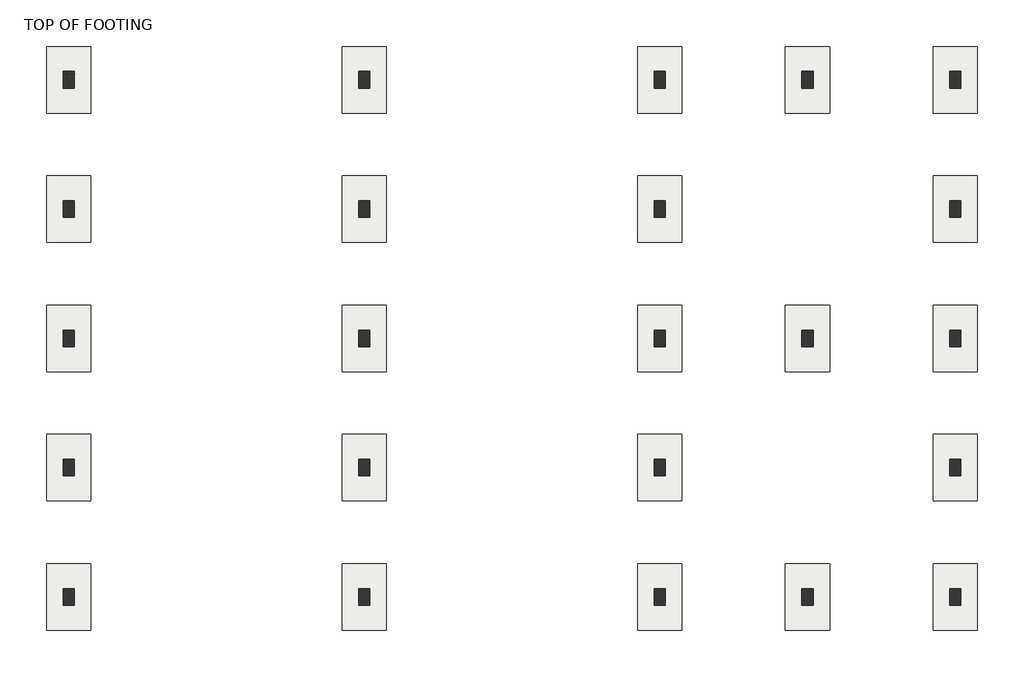
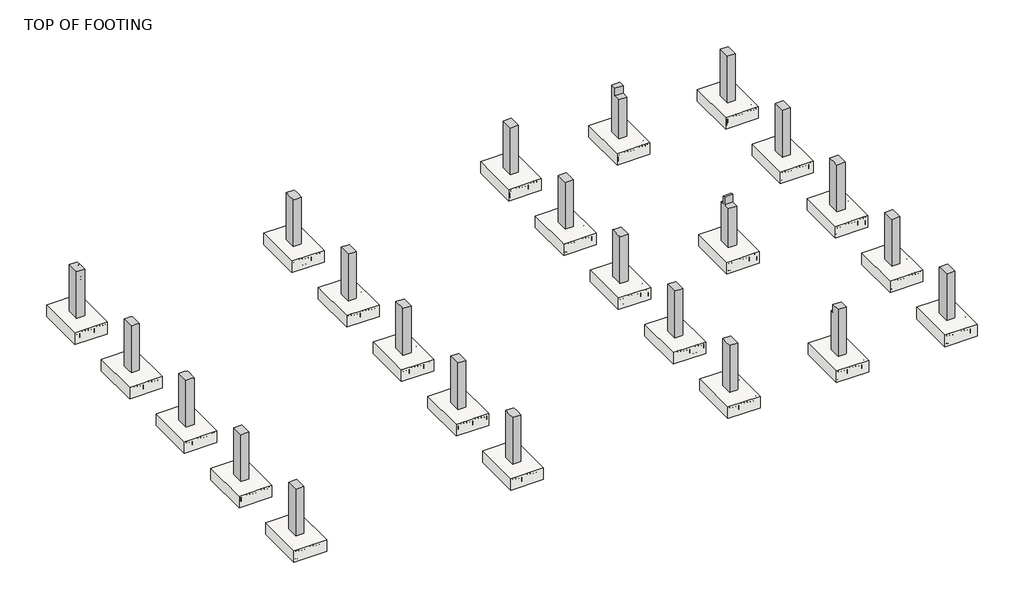
# One storey, part 1 of 8: 23 columns, 23 slabs.
"""IFC4 building model written with IfcOpenShell, lengths in millimetres."""

from ifc_helpers import new_model, si_unit, frame, origin, place, context, project, spatial, polyline, outline, extrude, faceted_brep, transform, mapped, element, save
from components import m_footing_rectangular_1800_x_1200_x_450mm_16ba7ea5

model = new_model("IFC4")

# Units and contexts
model_context = context("Model", 3, world=origin())
ifc_project = project(units=[si_unit("LENGTHUNIT", "METRE", prefix="MILLI")], contexts=[model_context])

# Site, building, storey
site = spatial("IfcSite", under=ifc_project)
building = spatial("IfcBuilding", under=site)
storey = spatial("IfcBuildingStorey", under=building, Name="TOP OF FOOTING", Elevation=-1828.8)

# Columns
placement = place(None, origin())
element("IfcColumn", 1, ObjectType="M_Concrete-Rectangular-Column : 300 x 450mm", at=placement, inside=storey, context=model_context, shape_type="Brep", body=[
    faceted_brep([(-11680.6874017, 15997.7008557, -1828.8), (-11680.6874017, 15547.7008557, -1828.8), (-11980.6874017, 15547.7008557, -1828.8), (-11980.6874017, 15997.7008557, -1828.8), (-11680.6874017, 15997.7008557, 0.0), (-11680.6874017, 15797.7008557, 0.0), (-11680.6874017, 15547.7008557, 0.0), (-11680.6874017, 15547.7008557, -300.0), (-11780.6874017, 15547.7008557, 0.0), (-11980.6874017, 15547.7008557, 0.0), (-11980.6874017, 15997.7008557, 0.0)], [[[0, 1, 2, 3]], [[1, 0, 4, 5, 6, 7]], [[2, 1, 7, 6, 8, 9]], [[3, 2, 9, 10]], [[0, 3, 10, 4]], [[10, 9, 8, 6, 5, 4]]]),
])
element("IfcColumn", 2, ObjectType="M_Concrete-Rectangular-Column : 300 x 450mm", at=placement, inside=storey, context=model_context, shape_type="Brep", body=[
    faceted_brep([(-11680.6874017, 8997.7008557, -1828.8), (-11680.6874017, 8547.7008557, -1828.8), (-11980.6874017, 8547.7008557, -1828.8), (-11980.6874017, 8997.7008557, -1828.8), (-11680.6874017, 8997.7008557, -300.0), (-11680.6874017, 8997.7008557, 0.0), (-11680.6874017, 8872.7008557, 0.0), (-11680.6874017, 8672.7008557, 0.0), (-11680.6874017, 8547.7008557, 0.0), (-11680.6874017, 8547.7008557, -300.0), (-11780.6874017, 8547.7008557, 0.0), (-11980.6874017, 8547.7008557, 0.0), (-11980.6874017, 8997.7008557, 0.0), (-11780.6874017, 8997.7008557, 0.0)], [[[0, 1, 2, 3]], [[1, 0, 4, 5, 6, 7, 8, 9]], [[2, 1, 9, 8, 10, 11]], [[3, 2, 11, 12]], [[0, 3, 12, 13, 5, 4]], [[12, 11, 10, 8, 7, 6, 5, 13]]]),
])
element("IfcColumn", 3, ObjectType="M_Concrete-Rectangular-Column : 300 x 450mm", at=placement, inside=storey, context=model_context, shape_type="Brep", body=[
    faceted_brep([(-11680.6874017, 1997.7008557, -1828.8), (-11680.6874017, 1547.7008557, -1828.8), (-11980.6874017, 1547.7008557, -1828.8), (-11980.6874017, 1997.7008557, -1828.8), (-11680.6874017, 1997.7008557, -300.0), (-11680.6874017, 1997.7008557, 0.0), (-11680.6874017, 1747.7008557, 0.0), (-11680.6874017, 1547.7008557, 0.0), (-11980.6874017, 1547.7008557, 0.0), (-11980.6874017, 1997.7008557, 0.0), (-11780.6874017, 1997.7008557, 0.0)], [[[0, 1, 2, 3]], [[1, 0, 4, 5, 6, 7]], [[2, 1, 7, 8]], [[3, 2, 8, 9]], [[0, 3, 9, 10, 5, 4]], [[8, 7, 6, 5, 10, 9]]]),
])
element("IfcColumn", 4, ObjectType="M_Concrete-Rectangular-Column : 300 x 450mm", at=placement, inside=storey, context=model_context, shape_type="Brep", body=[
    faceted_brep([(-3680.6874017, 15997.7008557, -1828.8), (-3680.6874017, 15547.7008557, -1828.8), (-3980.6874017, 15547.7008557, -1828.8), (-3980.6874017, 15997.7008557, -1828.8), (-3680.6874017, 15997.7008557, 0.0), (-3680.6874017, 15797.7008557, 0.0), (-3680.6874017, 15547.7008557, 0.0), (-3680.6874017, 15547.7008557, -300.0), (-3780.6874017, 15547.7008557, 0.0), (-3930.6874017, 15547.7008557, 0.0), (-3980.6874017, 15547.7008557, 0.0), (-3980.6874017, 15547.7008557, -300.0), (-3980.6874017, 15797.7008557, 0.0), (-3980.6874017, 15997.7008557, 0.0)], [[[0, 1, 2, 3]], [[1, 0, 4, 5, 6, 7]], [[2, 1, 7, 6, 8, 9, 10, 11]], [[3, 2, 11, 10, 12, 13]], [[0, 3, 13, 4]], [[4, 13, 12, 10, 9, 8, 6, 5]]]),
])
element("IfcColumn", 5, ObjectType="M_Concrete-Rectangular-Column : 300 x 450mm", at=placement, inside=storey, context=model_context, shape_type="Brep", body=[
    faceted_brep([(-3680.6874017, 12497.7008557, -1828.8), (-3680.6874017, 12047.7008557, -1828.8), (-3980.6874017, 12047.7008557, -1828.8), (-3980.6874017, 12497.7008557, -1828.8), (-3680.6874017, 12497.7008557, -300.0), (-3680.6874017, 12497.7008557, 0.0), (-3680.6874017, 12047.7008557, 0.0), (-3680.6874017, 12047.7008557, -300.0), (-3780.6874017, 12047.7008557, 0.0), (-3930.6874017, 12047.7008557, 0.0), (-3980.6874017, 12047.7008557, 0.0), (-3980.6874017, 12047.7008557, -300.0), (-3980.6874017, 12497.7008557, 0.0), (-3980.6874017, 12497.7008557, -300.0), (-3930.6874017, 12497.7008557, 0.0), (-3780.6874017, 12497.7008557, 0.0)], [[[0, 1, 2, 3]], [[1, 0, 4, 5, 6, 7]], [[2, 1, 7, 6, 8, 9, 10, 11]], [[3, 2, 11, 10, 12, 13]], [[0, 3, 13, 12, 14, 15, 5, 4]], [[6, 5, 15, 14, 12, 10, 9, 8]]]),
])
element("IfcColumn", 6, ObjectType="M_Concrete-Rectangular-Column : 300 x 450mm", at=placement, inside=storey, context=model_context, shape_type="Brep", body=[
    faceted_brep([(-3680.6874017, 8997.7008557, -1828.8), (-3680.6874017, 8547.7008557, -1828.8), (-3980.6874017, 8547.7008557, -1828.8), (-3980.6874017, 8997.7008557, -1828.8), (-3680.6874017, 8997.7008557, -300.0), (-3680.6874017, 8997.7008557, 0.0), (-3680.6874017, 8872.7008557, 0.0), (-3680.6874017, 8672.7008557, 0.0), (-3680.6874017, 8547.7008557, 0.0), (-3680.6874017, 8547.7008557, -300.0), (-3730.6874017, 8547.7008557, 0.0), (-3930.6874017, 8547.7008557, 0.0), (-3980.6874017, 8547.7008557, 0.0), (-3980.6874017, 8547.7008557, -300.0), (-3980.6874017, 8672.7008557, 0.0), (-3980.6874017, 8872.7008557, 0.0), (-3980.6874017, 8997.7008557, 0.0), (-3980.6874017, 8997.7008557, -300.0), (-3930.6874017, 8997.7008557, 0.0), (-3780.6874017, 8997.7008557, 0.0)], [[[0, 1, 2, 3]], [[1, 0, 4, 5, 6, 7, 8, 9]], [[2, 1, 9, 8, 10, 11, 12, 13]], [[3, 2, 13, 12, 14, 15, 16, 17]], [[0, 3, 17, 16, 18, 19, 5, 4]], [[18, 16, 15, 14, 12, 11, 10, 8, 7, 6, 5, 19]]]),
])
element("IfcColumn", 7, ObjectType="M_Concrete-Rectangular-Column : 300 x 450mm", at=placement, inside=storey, context=model_context, shape_type="Brep", body=[
    faceted_brep([(-3680.6874017, 5497.7008557, -1828.8), (-3680.6874017, 5047.7008557, -1828.8), (-3980.6874017, 5047.7008557, -1828.8), (-3980.6874017, 5497.7008557, -1828.8), (-3680.6874017, 5497.7008557, -300.0), (-3680.6874017, 5497.7008557, 0.0), (-3680.6874017, 5047.7008557, 0.0), (-3680.6874017, 5047.7008557, -300.0), (-3730.6874017, 5047.7008557, 0.0), (-3930.6874017, 5047.7008557, 0.0), (-3980.6874017, 5047.7008557, 0.0), (-3980.6874017, 5047.7008557, -300.0), (-3980.6874017, 5497.7008557, 0.0), (-3980.6874017, 5497.7008557, -300.0), (-3930.6874017, 5497.7008557, 0.0), (-3730.6874017, 5497.7008557, 0.0)], [[[0, 1, 2, 3]], [[1, 0, 4, 5, 6, 7]], [[2, 1, 7, 6, 8, 9, 10, 11]], [[3, 2, 11, 10, 12, 13]], [[0, 3, 13, 12, 14, 15, 5, 4]], [[6, 5, 15, 14, 12, 10, 9, 8]]]),
])
element("IfcColumn", 8, ObjectType="M_Concrete-Rectangular-Column : 300 x 450mm", at=placement, inside=storey, context=model_context, shape_type="Brep", body=[
    faceted_brep([(-3680.6874017, 1997.7008557, -1828.8), (-3680.6874017, 1547.7008557, -1828.8), (-3980.6874017, 1547.7008557, -1828.8), (-3980.6874017, 1997.7008557, -1828.8), (-3680.6874017, 1997.7008557, -300.0), (-3680.6874017, 1997.7008557, 0.0), (-3680.6874017, 1747.7008557, 0.0), (-3680.6874017, 1547.7008557, 0.0), (-3980.6874017, 1547.7008557, 0.0), (-3980.6874017, 1747.7008557, 0.0), (-3980.6874017, 1997.7008557, 0.0), (-3980.6874017, 1997.7008557, -300.0), (-3930.6874017, 1997.7008557, 0.0), (-3730.6874017, 1997.7008557, 0.0)], [[[0, 1, 2, 3]], [[1, 0, 4, 5, 6, 7]], [[2, 1, 7, 8]], [[3, 2, 8, 9, 10, 11]], [[0, 3, 11, 10, 12, 13, 5, 4]], [[8, 7, 6, 5, 13, 12, 10, 9]]]),
])
element("IfcColumn", 9, ObjectType="M_Concrete-Rectangular-Column : 300 x 450mm", at=placement, inside=storey, context=model_context, shape_type="Brep", body=[
    faceted_brep([(4319.3125983, 15997.7008557, -1828.8), (4319.3125983, 15547.7008557, -1828.8), (4019.3125983, 15547.7008557, -1828.8), (4019.3125983, 15997.7008557, -1828.8), (4319.3125983, 15997.7008557, 0.0), (4319.3125983, 15797.7008557, 0.0), (4319.3125983, 15547.7008557, 0.0), (4319.3125983, 15547.7008557, -300.0), (4219.3125983, 15547.7008557, 0.0), (4069.3125983, 15547.7008557, 0.0), (4019.3125983, 15547.7008557, 0.0), (4019.3125983, 15547.7008557, -300.0), (4019.3125983, 15797.7008557, 0.0), (4019.3125983, 15997.7008557, 0.0)], [[[0, 1, 2, 3]], [[1, 0, 4, 5, 6, 7]], [[2, 1, 7, 6, 8, 9, 10, 11]], [[3, 2, 11, 10, 12, 13]], [[0, 3, 13, 4]], [[4, 13, 12, 10, 9, 8, 6, 5]]]),
])
element("IfcColumn", 10, ObjectType="M_Concrete-Rectangular-Column : 300 x 450mm", at=placement, inside=storey, context=model_context, shape_type="Brep", body=[
    faceted_brep([(4319.3125983, 8997.7008557, -1828.8), (4319.3125983, 8547.7008557, -1828.8), (4019.3125983, 8547.7008557, -1828.8), (4019.3125983, 8997.7008557, -1828.8), (4319.3125983, 8997.7008557, -300.0), (4319.3125983, 8997.7008557, 0.0), (4319.3125983, 8872.7008557, 0.0), (4319.3125983, 8797.7008557, 0.0), (4319.3125983, 8547.7008557, 0.0), (4319.3125983, 8547.7008557, -300.0), (4219.3125983, 8547.7008557, 0.0), (4069.3125983, 8547.7008557, 0.0), (4019.3125983, 8547.7008557, 0.0), (4019.3125983, 8547.7008557, -300.0), (4019.3125983, 8672.7008557, 0.0), (4019.3125983, 8872.7008557, 0.0), (4019.3125983, 8997.7008557, 0.0), (4019.3125983, 8997.7008557, -300.0), (4069.3125983, 8997.7008557, 0.0), (4219.3125983, 8997.7008557, 0.0)], [[[0, 1, 2, 3]], [[1, 0, 4, 5, 6, 7, 8, 9]], [[2, 1, 9, 8, 10, 11, 12, 13]], [[3, 2, 13, 12, 14, 15, 16, 17]], [[0, 3, 17, 16, 18, 19, 5, 4]], [[18, 16, 15, 14, 12, 11, 10, 8, 7, 6, 5, 19]]]),
])
element("IfcColumn", 11, ObjectType="M_Concrete-Rectangular-Column : 300 x 450mm", at=placement, inside=storey, context=model_context, shape_type="Brep", body=[
    faceted_brep([(4319.3125983, 1997.7008557, -1828.8), (4319.3125983, 1547.7008557, -1828.8), (4019.3125983, 1547.7008557, -1828.8), (4019.3125983, 1997.7008557, -1828.8), (4319.3125983, 1997.7008557, -300.0), (4319.3125983, 1997.7008557, 0.0), (4319.3125983, 1872.7008557, 0.0), (4319.3125983, 1547.7008557, 0.0), (4019.3125983, 1547.7008557, 0.0), (4019.3125983, 1747.7008557, 0.0), (4019.3125983, 1997.7008557, 0.0), (4019.3125983, 1997.7008557, -300.0), (4069.3125983, 1997.7008557, 0.0), (4219.3125983, 1997.7008557, 0.0)], [[[0, 1, 2, 3]], [[1, 0, 4, 5, 6, 7]], [[2, 1, 7, 8]], [[3, 2, 8, 9, 10, 11]], [[0, 3, 11, 10, 12, 13, 5, 4]], [[8, 7, 6, 5, 13, 12, 10, 9]]]),
])
element("IfcColumn", 12, ObjectType="M_Concrete-Rectangular-Column : 300 x 450mm", at=placement, inside=storey, context=model_context, shape_type="SweptSolid", body=[
    extrude(outline(polyline([(15997.7008557, -1828.8), (15547.7008557, -1828.8), (15547.7008557, -300.0), (15797.7008557, -300.0), (15797.7008557, 0.0), (15997.7008557, 0.0), (15997.7008557, -1828.8)])), frame((8019.3125983, 0.0, 0.0), z_axis=(1.0, 0.0, 0.0), x_axis=(0.0, 1.0, 0.0)), (0.0, 0.0, 1.0), 300.0),
])
element("IfcColumn", 13, ObjectType="M_Concrete-Rectangular-Column : 300 x 450mm", at=placement, inside=storey, context=model_context, shape_type="SweptSolid", body=[
    extrude(outline(polyline([(1997.7008557, -1828.8), (1547.7008557, -1828.8), (1547.7008557, 0.0), (1872.7008557, 0.0), (1872.7008557, -300.0), (1997.7008557, -300.0), (1997.7008557, -1828.8)])), frame((8019.3125983, 0.0, 0.0), z_axis=(1.0, 0.0, 0.0), x_axis=(0.0, 1.0, 0.0)), (0.0, 0.0, 1.0), 300.0),
])
element("IfcColumn", 14, ObjectType="M_Concrete-Rectangular-Column : 300 x 450mm", at=placement, inside=storey, context=model_context, shape_type="Brep", body=[
    faceted_brep([(12319.3125983, 12497.7008557, -1828.8), (12319.3125983, 12047.7008557, -1828.8), (12019.3125983, 12047.7008557, -1828.8), (12019.3125983, 12497.7008557, -1828.8), (12319.3125983, 12497.7008557, 0.0), (12319.3125983, 12047.7008557, 0.0), (12069.3125983, 12047.7008557, 0.0), (12019.3125983, 12047.7008557, 0.0), (12019.3125983, 12047.7008557, -300.0), (12019.3125983, 12497.7008557, 0.0), (12019.3125983, 12497.7008557, -300.0), (12069.3125983, 12497.7008557, 0.0)], [[[0, 1, 2, 3]], [[1, 0, 4, 5]], [[2, 1, 5, 6, 7, 8]], [[3, 2, 8, 7, 9, 10]], [[0, 3, 10, 9, 11, 4]], [[5, 4, 11, 9, 7, 6]]]),
])
element("IfcColumn", 15, ObjectType="M_Concrete-Rectangular-Column : 300 x 450mm", at=placement, inside=storey, context=model_context, shape_type="Brep", body=[
    faceted_brep([(12319.3125983, 5497.7008557, -1828.8), (12319.3125983, 5047.7008557, -1828.8), (12019.3125983, 5047.7008557, -1828.8), (12019.3125983, 5497.7008557, -1828.8), (12319.3125983, 5497.7008557, 0.0), (12319.3125983, 5047.7008557, 0.0), (12069.3125983, 5047.7008557, 0.0), (12019.3125983, 5047.7008557, 0.0), (12019.3125983, 5047.7008557, -300.0), (12019.3125983, 5497.7008557, 0.0), (12019.3125983, 5497.7008557, -300.0), (12069.3125983, 5497.7008557, 0.0)], [[[0, 1, 2, 3]], [[1, 0, 4, 5]], [[2, 1, 5, 6, 7, 8]], [[3, 2, 8, 7, 9, 10]], [[0, 3, 10, 9, 11, 4]], [[5, 4, 11, 9, 7, 6]]]),
])
element("IfcColumn", 16, ObjectType="M_Concrete-Rectangular-Column : 300 x 450mm", at=placement, inside=storey, context=model_context, shape_type="Brep", body=[
    faceted_brep([(12319.3125983, 15997.7008557, -1828.8), (12319.3125983, 15547.7008557, -1828.8), (12019.3125983, 15547.7008557, -1828.8), (12019.3125983, 15997.7008557, -1828.8), (12319.3125983, 15997.7008557, 0.0), (12319.3125983, 15547.7008557, 0.0), (12069.3125983, 15547.7008557, 0.0), (12019.3125983, 15547.7008557, 0.0), (12019.3125983, 15547.7008557, -300.0), (12019.3125983, 15797.7008557, 0.0), (12019.3125983, 15997.7008557, 0.0)], [[[0, 1, 2, 3]], [[1, 0, 4, 5]], [[2, 1, 5, 6, 7, 8]], [[3, 2, 8, 7, 9, 10]], [[0, 3, 10, 4]], [[5, 4, 10, 9, 7, 6]]]),
])
element("IfcColumn", 17, ObjectType="M_Concrete-Rectangular-Column : 300 x 450mm", at=placement, inside=storey, context=model_context, shape_type="Brep", body=[
    faceted_brep([(12319.3125983, 1997.7008557, -1828.8), (12319.3125983, 1547.7008557, -1828.8), (12019.3125983, 1547.7008557, -1828.8), (12019.3125983, 1997.7008557, -1828.8), (12319.3125983, 1997.7008557, 0.0), (12319.3125983, 1547.7008557, 0.0), (12019.3125983, 1547.7008557, 0.0), (12019.3125983, 1872.7008557, 0.0), (12019.3125983, 1997.7008557, 0.0), (12019.3125983, 1997.7008557, -300.0), (12069.3125983, 1997.7008557, 0.0)], [[[0, 1, 2, 3]], [[1, 0, 4, 5]], [[2, 1, 5, 6]], [[3, 2, 6, 7, 8, 9]], [[0, 3, 9, 8, 10, 4]], [[5, 4, 10, 8, 7, 6]]]),
])
element("IfcColumn", 18, ObjectType="M_Concrete-Rectangular-Column : 300 x 450mm", at=placement, inside=storey, context=model_context, shape_type="Brep", body=[
    faceted_brep([(-11680.6874017, 12497.7008557, -1828.8), (-11680.6874017, 12047.7008557, -1828.8), (-11980.6874017, 12047.7008557, -1828.8), (-11980.6874017, 12497.7008557, -1828.8), (-11680.6874017, 12497.7008557, -300.0), (-11680.6874017, 12497.7008557, 0.0), (-11680.6874017, 12047.7008557, 0.0), (-11680.6874017, 12047.7008557, -300.0), (-11780.6874017, 12047.7008557, 0.0), (-11980.6874017, 12047.7008557, 0.0), (-11980.6874017, 12497.7008557, 0.0), (-11780.6874017, 12497.7008557, 0.0)], [[[0, 1, 2, 3]], [[1, 0, 4, 5, 6, 7]], [[2, 1, 7, 6, 8, 9]], [[3, 2, 9, 10]], [[0, 3, 10, 11, 5, 4]], [[6, 5, 11, 10, 9, 8]]]),
])
element("IfcColumn", 19, ObjectType="M_Concrete-Rectangular-Column : 300 x 450mm", at=placement, inside=storey, context=model_context, shape_type="Brep", body=[
    faceted_brep([(-11680.6874017, 5497.7008557, -1828.8), (-11680.6874017, 5047.7008557, -1828.8), (-11980.6874017, 5047.7008557, -1828.8), (-11980.6874017, 5497.7008557, -1828.8), (-11680.6874017, 5497.7008557, -300.0), (-11680.6874017, 5497.7008557, 0.0), (-11680.6874017, 5047.7008557, 0.0), (-11680.6874017, 5047.7008557, -300.0), (-11780.6874017, 5047.7008557, 0.0), (-11980.6874017, 5047.7008557, 0.0), (-11980.6874017, 5497.7008557, 0.0), (-11780.6874017, 5497.7008557, 0.0)], [[[0, 1, 2, 3]], [[1, 0, 4, 5, 6, 7]], [[2, 1, 7, 6, 8, 9]], [[3, 2, 9, 10]], [[0, 3, 10, 11, 5, 4]], [[6, 5, 11, 10, 9, 8]]]),
])
element("IfcColumn", 20, ObjectType="M_Concrete-Rectangular-Column : 300 x 450mm", at=placement, inside=storey, context=model_context, shape_type="Brep", body=[
    faceted_brep([(12319.3125983, 8997.7008557, -1828.8), (12319.3125983, 8547.7008557, -1828.8), (12019.3125983, 8547.7008557, -1828.8), (12019.3125983, 8997.7008557, -1828.8), (12319.3125983, 8997.7008557, 0.0), (12319.3125983, 8547.7008557, 0.0), (12069.3125983, 8547.7008557, 0.0), (12019.3125983, 8547.7008557, 0.0), (12019.3125983, 8547.7008557, -300.0), (12019.3125983, 8797.7008557, 0.0), (12019.3125983, 8872.7008557, 0.0), (12019.3125983, 8997.7008557, 0.0), (12019.3125983, 8997.7008557, -300.0), (12069.3125983, 8997.7008557, 0.0)], [[[0, 1, 2, 3]], [[1, 0, 4, 5]], [[2, 1, 5, 6, 7, 8]], [[3, 2, 8, 7, 9, 10, 11, 12]], [[0, 3, 12, 11, 13, 4]], [[5, 4, 13, 11, 10, 9, 7, 6]]]),
])
element("IfcColumn", 21, ObjectType="M_Concrete-Rectangular-Column : 300 x 450mm", at=placement, inside=storey, context=model_context, shape_type="Brep", body=[
    faceted_brep([(8319.3125983, 8997.7008557, -1828.8), (8319.3125983, 8547.7008557, -1828.8), (8019.3125983, 8547.7008557, -1828.8), (8019.3125983, 8997.7008557, -1828.8), (8319.3125983, 8997.7008557, -300.0), (8319.3125983, 8872.7008557, -300.0), (8319.3125983, 8872.7008557, 0.0), (8319.3125983, 8797.7008557, 0.0), (8319.3125983, 8797.7008557, -300.0), (8319.3125983, 8547.7008557, -300.0), (8019.3125983, 8547.7008557, -300.0), (8019.3125983, 8672.7008557, -300.0), (8019.3125983, 8797.7008557, -300.0), (8019.3125983, 8797.7008557, 0.0), (8019.3125983, 8872.7008557, 0.0), (8019.3125983, 8872.7008557, -300.0), (8019.3125983, 8997.7008557, -300.0)], [[[0, 1, 2, 3]], [[1, 0, 4, 5, 6, 7, 8, 9]], [[2, 1, 9, 10]], [[3, 2, 10, 11, 12, 13, 14, 15, 16]], [[0, 3, 16, 4]], [[14, 13, 7, 6]], [[8, 12, 11, 10, 9]], [[5, 15, 14, 6]], [[12, 8, 7, 13]], [[15, 5, 4, 16]]]),
])
element("IfcColumn", 22, ObjectType="M_Concrete-Rectangular-Column : 300 x 450mm", at=placement, inside=storey, context=model_context, shape_type="Brep", body=[
    faceted_brep([(4319.3125983, 12497.7008557, -1828.8), (4319.3125983, 12047.7008557, -1828.8), (4019.3125983, 12047.7008557, -1828.8), (4019.3125983, 12497.7008557, -1828.8), (4319.3125983, 12497.7008557, -300.0), (4319.3125983, 12497.7008557, 0.0), (4319.3125983, 12047.7008557, 0.0), (4319.3125983, 12047.7008557, -300.0), (4219.3125983, 12047.7008557, 0.0), (4069.3125983, 12047.7008557, 0.0), (4019.3125983, 12047.7008557, 0.0), (4019.3125983, 12047.7008557, -300.0), (4019.3125983, 12497.7008557, 0.0), (4019.3125983, 12497.7008557, -300.0), (4069.3125983, 12497.7008557, 0.0), (4219.3125983, 12497.7008557, 0.0)], [[[0, 1, 2, 3]], [[1, 0, 4, 5, 6, 7]], [[2, 1, 7, 6, 8, 9, 10, 11]], [[3, 2, 11, 10, 12, 13]], [[0, 3, 13, 12, 14, 15, 5, 4]], [[6, 5, 15, 14, 12, 10, 9, 8]]]),
])
element("IfcColumn", 23, ObjectType="M_Concrete-Rectangular-Column : 300 x 450mm", at=placement, inside=storey, context=model_context, shape_type="Brep", body=[
    faceted_brep([(4319.3125983, 5497.7008557, -1828.8), (4319.3125983, 5047.7008557, -1828.8), (4019.3125983, 5047.7008557, -1828.8), (4019.3125983, 5497.7008557, -1828.8), (4319.3125983, 5497.7008557, -300.0), (4319.3125983, 5497.7008557, 0.0), (4319.3125983, 5047.7008557, 0.0), (4319.3125983, 5047.7008557, -300.0), (4219.3125983, 5047.7008557, 0.0), (4069.3125983, 5047.7008557, 0.0), (4019.3125983, 5047.7008557, 0.0), (4019.3125983, 5047.7008557, -300.0), (4019.3125983, 5497.7008557, 0.0), (4019.3125983, 5497.7008557, -300.0), (4069.3125983, 5497.7008557, 0.0), (4219.3125983, 5497.7008557, 0.0)], [[[0, 1, 2, 3]], [[1, 0, 4, 5, 6, 7]], [[2, 1, 7, 6, 8, 9, 10, 11]], [[3, 2, 11, 10, 12, 13]], [[0, 3, 13, 12, 14, 15, 5, 4]], [[6, 5, 15, 14, 12, 10, 9, 8]]]),
])

# Slabs
m_footing_rectangular_1800_x_1200_x_450mm_shape = m_footing_rectangular_1800_x_1200_x_450mm_16ba7ea5(model_context)
element("IfcSlab", 24, ObjectType="M_Footing-Rectangular : 1800 x 1200 x 450mm", at=placement, inside=storey, context=model_context, shape_type="MappedRepresentation", body=[
    mapped(m_footing_rectangular_1800_x_1200_x_450mm_shape, transform((-11830.6874017, 15772.7008557, -1828.8), x_axis=(1.0, 0.0, 0.0), y_axis=(0.0, 1.0, 0.0), z_axis=(0.0, 0.0, 1.0))),
])
element("IfcSlab", 25, ObjectType="M_Footing-Rectangular : 1800 x 1200 x 450mm", at=placement, inside=storey, context=model_context, shape_type="MappedRepresentation", body=[
    mapped(m_footing_rectangular_1800_x_1200_x_450mm_shape, transform((-11830.6874017, 8772.7008557, -1828.8), x_axis=(1.0, 0.0, 0.0), y_axis=(0.0, 1.0, 0.0), z_axis=(0.0, 0.0, 1.0))),
])
element("IfcSlab", 26, ObjectType="M_Footing-Rectangular : 1800 x 1200 x 450mm", at=placement, inside=storey, context=model_context, shape_type="MappedRepresentation", body=[
    mapped(m_footing_rectangular_1800_x_1200_x_450mm_shape, transform((-11830.6874017, 1772.7008557, -1828.8), x_axis=(1.0, 0.0, 0.0), y_axis=(0.0, 1.0, 0.0), z_axis=(0.0, 0.0, 1.0))),
])
element("IfcSlab", 27, ObjectType="M_Footing-Rectangular : 1800 x 1200 x 450mm", at=placement, inside=storey, context=model_context, shape_type="MappedRepresentation", body=[
    mapped(m_footing_rectangular_1800_x_1200_x_450mm_shape, transform((-3830.6874017, 15772.7008557, -1828.8), x_axis=(1.0, 0.0, 0.0), y_axis=(0.0, 1.0, 0.0), z_axis=(0.0, 0.0, 1.0))),
])
element("IfcSlab", 28, ObjectType="M_Footing-Rectangular : 1800 x 1200 x 450mm", at=placement, inside=storey, context=model_context, shape_type="MappedRepresentation", body=[
    mapped(m_footing_rectangular_1800_x_1200_x_450mm_shape, transform((-3830.6874017, 8772.7008557, -1828.8), x_axis=(1.0, 0.0, 0.0), y_axis=(0.0, 1.0, 0.0), z_axis=(0.0, 0.0, 1.0))),
])
element("IfcSlab", 29, ObjectType="M_Footing-Rectangular : 1800 x 1200 x 450mm", at=placement, inside=storey, context=model_context, shape_type="MappedRepresentation", body=[
    mapped(m_footing_rectangular_1800_x_1200_x_450mm_shape, transform((-3830.6874017, 1772.7008557, -1828.8), x_axis=(1.0, 0.0, 0.0), y_axis=(0.0, 1.0, 0.0), z_axis=(0.0, 0.0, 1.0))),
])
element("IfcSlab", 30, ObjectType="M_Footing-Rectangular : 1800 x 1200 x 450mm", at=placement, inside=storey, context=model_context, shape_type="MappedRepresentation", body=[
    mapped(m_footing_rectangular_1800_x_1200_x_450mm_shape, transform((4169.3125983, 15772.7008557, -1828.8), x_axis=(1.0, 0.0, 0.0), y_axis=(0.0, 1.0, 0.0), z_axis=(0.0, 0.0, 1.0))),
])
element("IfcSlab", 31, ObjectType="M_Footing-Rectangular : 1800 x 1200 x 450mm", at=placement, inside=storey, context=model_context, shape_type="MappedRepresentation", body=[
    mapped(m_footing_rectangular_1800_x_1200_x_450mm_shape, transform((4169.3125983, 8772.7008557, -1828.8), x_axis=(1.0, 0.0, 0.0), y_axis=(0.0, 1.0, 0.0), z_axis=(0.0, 0.0, 1.0))),
])
element("IfcSlab", 32, ObjectType="M_Footing-Rectangular : 1800 x 1200 x 450mm", at=placement, inside=storey, context=model_context, shape_type="MappedRepresentation", body=[
    mapped(m_footing_rectangular_1800_x_1200_x_450mm_shape, transform((4169.3125983, 1772.7008557, -1828.8), x_axis=(1.0, 0.0, 0.0), y_axis=(0.0, 1.0, 0.0), z_axis=(0.0, 0.0, 1.0))),
])
element("IfcSlab", 33, ObjectType="M_Footing-Rectangular : 1800 x 1200 x 450mm", at=placement, inside=storey, context=model_context, shape_type="MappedRepresentation", body=[
    mapped(m_footing_rectangular_1800_x_1200_x_450mm_shape, transform((8169.3125983, 15772.7008557, -1828.8), x_axis=(1.0, 0.0, 0.0), y_axis=(0.0, 1.0, 0.0), z_axis=(0.0, 0.0, 1.0))),
])
element("IfcSlab", 34, ObjectType="M_Footing-Rectangular : 1800 x 1200 x 450mm", at=placement, inside=storey, context=model_context, shape_type="MappedRepresentation", body=[
    mapped(m_footing_rectangular_1800_x_1200_x_450mm_shape, transform((8169.3125983, 1772.7008557, -1828.8), x_axis=(1.0, 0.0, 0.0), y_axis=(0.0, 1.0, 0.0), z_axis=(0.0, 0.0, 1.0))),
])
element("IfcSlab", 35, ObjectType="M_Footing-Rectangular : 1800 x 1200 x 450mm", at=placement, inside=storey, context=model_context, shape_type="MappedRepresentation", body=[
    mapped(m_footing_rectangular_1800_x_1200_x_450mm_shape, transform((12169.3125983, 12272.7008557, -1828.8), x_axis=(1.0, 0.0, 0.0), y_axis=(0.0, 1.0, 0.0), z_axis=(0.0, 0.0, 1.0))),
])
element("IfcSlab", 36, ObjectType="M_Footing-Rectangular : 1800 x 1200 x 450mm", at=placement, inside=storey, context=model_context, shape_type="MappedRepresentation", body=[
    mapped(m_footing_rectangular_1800_x_1200_x_450mm_shape, transform((12169.3125983, 5272.7008557, -1828.8), x_axis=(1.0, 0.0, 0.0), y_axis=(0.0, 1.0, 0.0), z_axis=(0.0, 0.0, 1.0))),
])
element("IfcSlab", 37, ObjectType="M_Footing-Rectangular : 1800 x 1200 x 450mm", at=placement, inside=storey, context=model_context, shape_type="MappedRepresentation", body=[
    mapped(m_footing_rectangular_1800_x_1200_x_450mm_shape, transform((12169.3125983, 15772.7008557, -1828.8), x_axis=(1.0, 0.0, 0.0), y_axis=(0.0, 1.0, 0.0), z_axis=(0.0, 0.0, 1.0))),
])
element("IfcSlab", 38, ObjectType="M_Footing-Rectangular : 1800 x 1200 x 450mm", at=placement, inside=storey, context=model_context, shape_type="MappedRepresentation", body=[
    mapped(m_footing_rectangular_1800_x_1200_x_450mm_shape, transform((12169.3125983, 1772.7008557, -1828.8), x_axis=(1.0, 0.0, 0.0), y_axis=(0.0, 1.0, 0.0), z_axis=(0.0, 0.0, 1.0))),
])
element("IfcSlab", 39, ObjectType="M_Footing-Rectangular : 1800 x 1200 x 450mm", at=placement, inside=storey, context=model_context, shape_type="MappedRepresentation", body=[
    mapped(m_footing_rectangular_1800_x_1200_x_450mm_shape, transform((12169.3125983, 8772.7008557, -1828.8), x_axis=(1.0, 0.0, 0.0), y_axis=(0.0, 1.0, 0.0), z_axis=(0.0, 0.0, 1.0))),
])
element("IfcSlab", 40, ObjectType="M_Footing-Rectangular : 1800 x 1200 x 450mm", at=placement, inside=storey, context=model_context, shape_type="MappedRepresentation", body=[
    mapped(m_footing_rectangular_1800_x_1200_x_450mm_shape, transform((-11830.6874017, 5272.7008557, -1828.8), x_axis=(1.0, 0.0, 0.0), y_axis=(0.0, 1.0, 0.0), z_axis=(0.0, 0.0, 1.0))),
])
element("IfcSlab", 41, ObjectType="M_Footing-Rectangular : 1800 x 1200 x 450mm", at=placement, inside=storey, context=model_context, shape_type="MappedRepresentation", body=[
    mapped(m_footing_rectangular_1800_x_1200_x_450mm_shape, transform((-11830.6874017, 12272.7008557, -1828.8), x_axis=(1.0, 0.0, 0.0), y_axis=(0.0, 1.0, 0.0), z_axis=(0.0, 0.0, 1.0))),
])
element("IfcSlab", 42, ObjectType="M_Footing-Rectangular : 1800 x 1200 x 450mm", at=placement, inside=storey, context=model_context, shape_type="MappedRepresentation", body=[
    mapped(m_footing_rectangular_1800_x_1200_x_450mm_shape, transform((-3830.6874017, 12272.7008557, -1828.8), x_axis=(1.0, 0.0, 0.0), y_axis=(0.0, 1.0, 0.0), z_axis=(0.0, 0.0, 1.0))),
])
element("IfcSlab", 43, ObjectType="M_Footing-Rectangular : 1800 x 1200 x 450mm", at=placement, inside=storey, context=model_context, shape_type="MappedRepresentation", body=[
    mapped(m_footing_rectangular_1800_x_1200_x_450mm_shape, transform((8169.3125983, 8772.7008557, -1828.8), x_axis=(1.0, 0.0, 0.0), y_axis=(0.0, 1.0, 0.0), z_axis=(0.0, 0.0, 1.0))),
])
element("IfcSlab", 44, ObjectType="M_Footing-Rectangular : 1800 x 1200 x 450mm", at=placement, inside=storey, context=model_context, shape_type="MappedRepresentation", body=[
    mapped(m_footing_rectangular_1800_x_1200_x_450mm_shape, transform((-3830.6874017, 5272.7008557, -1828.8), x_axis=(1.0, 0.0, 0.0), y_axis=(0.0, 1.0, 0.0), z_axis=(0.0, 0.0, 1.0))),
])
element("IfcSlab", 45, ObjectType="M_Footing-Rectangular : 1800 x 1200 x 450mm", at=placement, inside=storey, context=model_context, shape_type="MappedRepresentation", body=[
    mapped(m_footing_rectangular_1800_x_1200_x_450mm_shape, transform((4169.3125983, 5272.7008557, -1828.8), x_axis=(1.0, 0.0, 0.0), y_axis=(0.0, 1.0, 0.0), z_axis=(0.0, 0.0, 1.0))),
])
element("IfcSlab", 46, ObjectType="M_Footing-Rectangular : 1800 x 1200 x 450mm", at=placement, inside=storey, context=model_context, shape_type="MappedRepresentation", body=[
    mapped(m_footing_rectangular_1800_x_1200_x_450mm_shape, transform((4169.3125983, 12272.7008557, -1828.8), x_axis=(1.0, 0.0, 0.0), y_axis=(0.0, 1.0, 0.0), z_axis=(0.0, 0.0, 1.0))),
])

save(model, "model.ifc")

# Revit data of these elements
# Grids (mm)
#   "1": line (-11830.687, 18195.955) -> (-11830.687, -10806.418)
#   "2": line (-7830.687, 18195.955) -> (-7830.687, -10806.418)
#   "3": line (-3830.687, 18195.955) -> (-3830.687, -10806.418)
#   "4": line (169.313, 18195.955) -> (169.313, -10806.418)
#   "5": line (4169.313, 18195.955) -> (4169.313, -10806.418)
#   "6": line (8169.313, 18195.955) -> (8169.313, -10806.418)
#   "A": line (19604.118, 15772.701) -> (-13472.277, 15772.701)
#   "B": line (19604.118, 12272.701) -> (-13472.277, 12272.701)
#   "C": line (19604.118, 8772.701) -> (-13472.277, 8772.701)
#   "D": line (19604.118, 5272.701) -> (-13472.277, 5272.701)
#   "E": line (19604.118, 1772.701) -> (-13472.277, 1772.701)
#   "F": line (12169.313, 18195.955) -> (12169.313, -10806.418)
# Type "M_Concrete-Rectangular-Column : 300 x 450mm"
#   b = 0' - 11.81102"
#   h = 1' - 5.71654"
#   Structural Material [instance default] = Concrete, Cast-in-Place gray
# Type "M_Footing-Rectangular : 1800 x 1200 x 450mm"
#   Width = 3' - 11.24409"
#   Length = 5' - 10.86614"
#   Foundation Thickness = 1' - 5.71654"
#   Structural Material [instance default] = Concrete, Cast-in-Place gray
#   Assembly Code = ""
# Elements 1, 2, 3, 4, 5, 6, 7, 8, 9, 10, 11, 12, 13, 14, 15, 16, 17, 18, 19, 20, 21, 22, 23 (IfcColumn, "M_Concrete-Rectangular-Column : 300 x 450mm")
#   Structural Material = Concrete, Cast-in-Place gray
#   Phase Created = New Construction
#   Materials on its faces: "Concrete, Cast-in-Place gray"
# Elements 24, 25, 26, 27, 28, 29, 30, 31, 32, 33, 34, 35, 36, 37, 38, 39, 40, 41, 42, 43, 44, 45, 46 (IfcSlab, "M_Footing-Rectangular : 1800 x 1200 x 450mm")
#   Structural Material = Concrete, Cast-in-Place gray
#   Phase Created = New Construction
#   Materials on its faces: "Concrete, Cast-in-Place gray"
# Materials
#   "Concrete, Cast-in-Place gray": class "Concrete", colour RGB 192 192 192, transparency 0, Description = "Cast-in-place concrete", Cost = 0
